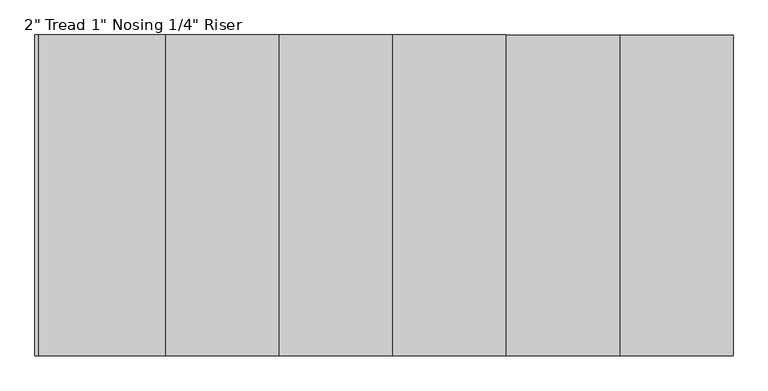
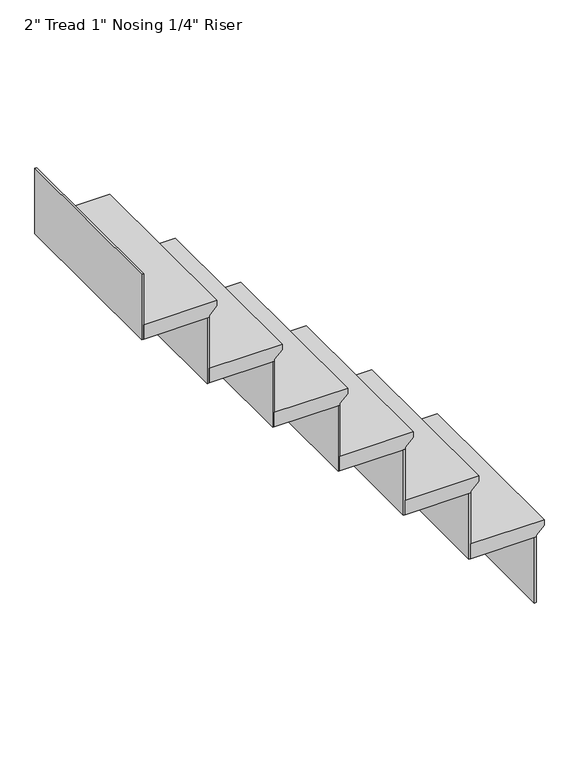
"""IFC4 building model written with IfcOpenShell, lengths in millimetres: stair flight geometry."""

from ifc_helpers import new_model, si_unit, frame, origin, place, context, project, spatial, polyline, outline, extrude, source, transform, mapped, element, save


def stair_flight_15f1c366(model_context):
    return source(origin(), model_context, "Body", "SweptSolid", [
        extrude(outline(polyline([(1828.8, -3296.0237097), (1828.8, -3537.3237097), (1778.0, -3537.3237097), (1778.0, -3321.4237097), (1784.35, -3321.4237097), (1809.75, -3296.0237097), (1828.8, -3296.0237097)])), frame((0.0, 4341.1083475, 0.0), z_axis=(0.0, 1.0, 0.0), x_axis=(0.0, 0.0, 1.0)), (0.0, 0.0, 1.0), 609.6),
        extrude(outline(polyline([(-3327.7737097, 4950.7083475), (-3321.4237097, 4950.7083475), (-3321.4237097, 4341.1083475), (-3327.7737097, 4341.1083475), (-3327.7737097, 4950.7083475)])), frame((0.0, 0.0, 1549.4), z_axis=(0.0, 0.0, 1.0), x_axis=(1.0, 0.0, 0.0)), (0.0, 0.0, 1.0), 228.6),
        extrude(outline(polyline([(-4623.1737097, 4950.7083475), (-4616.8237097, 4950.7083475), (-4616.8237097, 4341.1083475), (-4623.1737097, 4341.1083475), (-4623.1737097, 4950.7083475)])), frame((0.0, 0.0, 2921.0), z_axis=(0.0, 0.0, 1.0), x_axis=(1.0, 0.0, 0.0)), (0.0, 0.0, 1.0), 228.6),
        extrude(outline(polyline([(-3543.6737097, 4950.7083475), (-3537.3237097, 4950.7083475), (-3537.3237097, 4341.1083475), (-3543.6737097, 4341.1083475), (-3543.6737097, 4950.7083475)])), frame((0.0, 0.0, 1778.0), z_axis=(0.0, 0.0, 1.0), x_axis=(1.0, 0.0, 0.0)), (0.0, 0.0, 1.0), 228.6),
        extrude(outline(polyline([(2057.4, -3511.9237097), (2057.4, -3753.2237097), (2006.6, -3753.2237097), (2006.6, -3537.3237097), (2012.95, -3537.3237097), (2038.35, -3511.9237097), (2057.4, -3511.9237097)])), frame((0.0, 4341.1083475, 0.0), z_axis=(0.0, 1.0, 0.0), x_axis=(0.0, 0.0, 1.0)), (0.0, 0.0, 1.0), 609.6),
        extrude(outline(polyline([(-3759.5737097, 4950.7083475), (-3753.2237097, 4950.7083475), (-3753.2237097, 4341.1083475), (-3759.5737097, 4341.1083475), (-3759.5737097, 4950.7083475)])), frame((0.0, 0.0, 2006.6), z_axis=(0.0, 0.0, 1.0), x_axis=(1.0, 0.0, 0.0)), (0.0, 0.0, 1.0), 228.6),
        extrude(outline(polyline([(2286.0, -3727.8237097), (2286.0, -3969.1237097), (2235.2, -3969.1237097), (2235.2, -3753.2237097), (2241.55, -3753.2237097), (2266.95, -3727.8237097), (2286.0, -3727.8237097)])), frame((0.0, 4341.1083475, 0.0), z_axis=(0.0, 1.0, 0.0), x_axis=(0.0, 0.0, 1.0)), (0.0, 0.0, 1.0), 609.6),
        extrude(outline(polyline([(-3975.4737097, 4950.7083475), (-3969.1237097, 4950.7083475), (-3969.1237097, 4341.1083475), (-3975.4737097, 4341.1083475), (-3975.4737097, 4950.7083475)])), frame((0.0, 0.0, 2235.2), z_axis=(0.0, 0.0, 1.0), x_axis=(1.0, 0.0, 0.0)), (0.0, 0.0, 1.0), 228.6),
        extrude(outline(polyline([(2514.6, -3943.7237097), (2514.6, -4185.0237097), (2463.8, -4185.0237097), (2463.8, -3969.1237097), (2470.15, -3969.1237097), (2495.55, -3943.7237097), (2514.6, -3943.7237097)])), frame((0.0, 4341.1083475, 0.0), z_axis=(0.0, 1.0, 0.0), x_axis=(0.0, 0.0, 1.0)), (0.0, 0.0, 1.0), 609.6),
        extrude(outline(polyline([(-4191.3737097, 4950.7083475), (-4185.0237097, 4950.7083475), (-4185.0237097, 4341.1083475), (-4191.3737097, 4341.1083475), (-4191.3737097, 4950.7083475)])), frame((0.0, 0.0, 2463.8), z_axis=(0.0, 0.0, 1.0), x_axis=(1.0, 0.0, 0.0)), (0.0, 0.0, 1.0), 228.6),
        extrude(outline(polyline([(2743.2, -4159.6237097), (2743.2, -4400.9237097), (2692.4, -4400.9237097), (2692.4, -4185.0237097), (2698.75, -4185.0237097), (2724.15, -4159.6237097), (2743.2, -4159.6237097)])), frame((0.0, 4341.1083475, 0.0), z_axis=(0.0, 1.0, 0.0), x_axis=(0.0, 0.0, 1.0)), (0.0, 0.0, 1.0), 609.6),
        extrude(outline(polyline([(-4407.2737097, 4950.7083475), (-4400.9237097, 4950.7083475), (-4400.9237097, 4341.1083475), (-4407.2737097, 4341.1083475), (-4407.2737097, 4950.7083475)])), frame((0.0, 0.0, 2692.4), z_axis=(0.0, 0.0, 1.0), x_axis=(1.0, 0.0, 0.0)), (0.0, 0.0, 1.0), 228.6),
        extrude(outline(polyline([(2971.8, -4375.5237097), (2971.8, -4616.8237097), (2921.0, -4616.8237097), (2921.0, -4400.9237097), (2927.35, -4400.9237097), (2952.75, -4375.5237097), (2971.8, -4375.5237097)])), frame((0.0, 4341.1083475, 0.0), z_axis=(0.0, 1.0, 0.0), x_axis=(0.0, 0.0, 1.0)), (0.0, 0.0, 1.0), 609.6),
    ])


if __name__ == "__main__":
    model = new_model("IFC4")
    model_context = context("Model", 3, world=origin())
    ifc_project = project(units=[si_unit("LENGTHUNIT", "METRE", prefix="MILLI")], contexts=[model_context])
    site = spatial("IfcSite", under=ifc_project)
    building = spatial("IfcBuilding", under=site)
    placement = place(None, origin())
    stair_flight_shape = stair_flight_15f1c366(model_context)
    element("IfcStairFlight", 1, ObjectType="2\" Tread 1\" Nosing 1/4\" Riser", at=placement, inside=building, context=model_context, shape_type="MappedRepresentation", body=[
        mapped(stair_flight_shape, transform((0.0, 0.0, 0.0), x_axis=(1.0, 0.0, 0.0), y_axis=(0.0, 1.0, 0.0), z_axis=(0.0, 0.0, 1.0))),
    ])
    save(model, "model.ifc")
